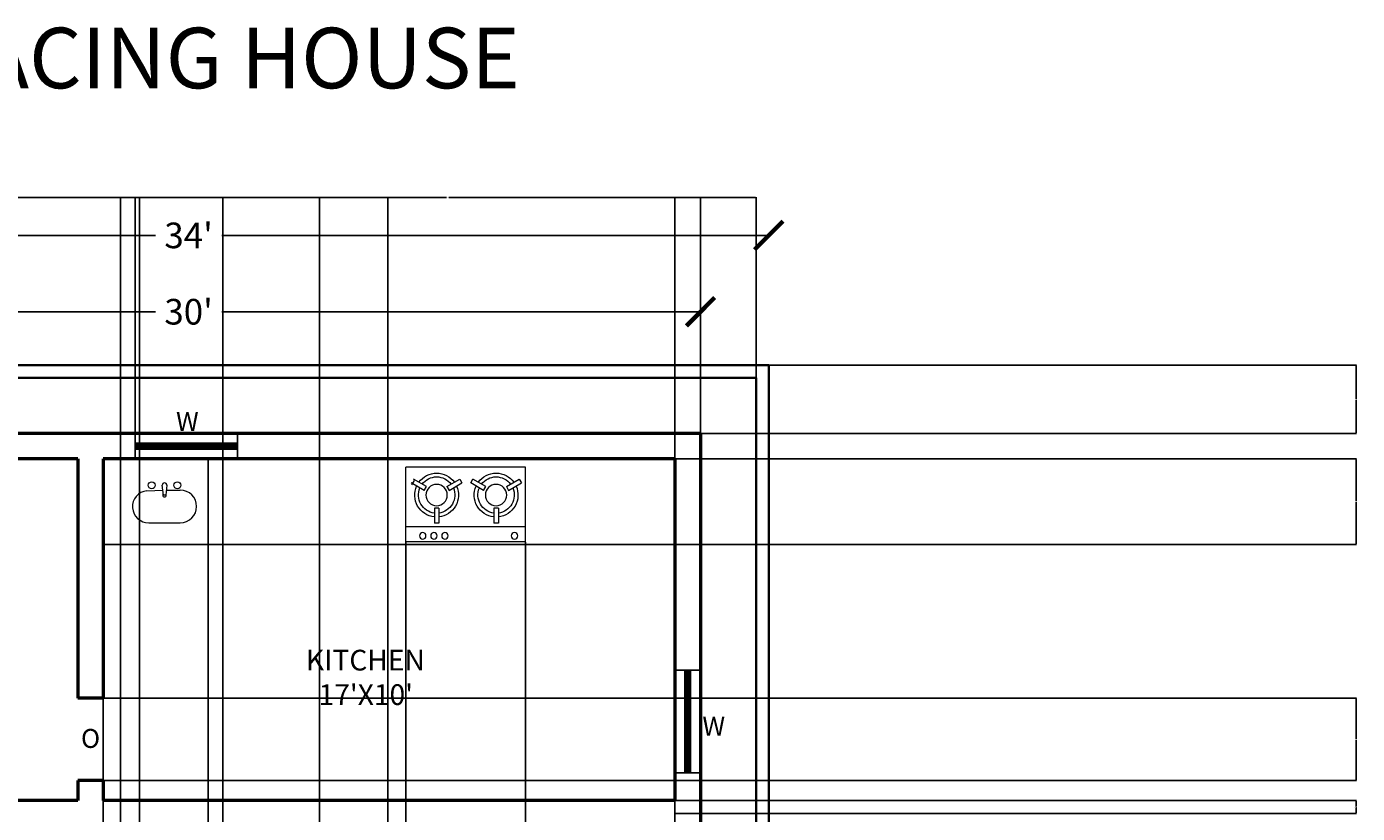
# Model space of a CAD drawing. Units: inches. Extents: x 338 to 1188, y -996 to 127.
# Tile 15 of 15: x 720 to 1188, y -149 to 127. Entities that reach past the tile are written whole.
import ezdxf

# ---------------------------------------------------------------- set-up
doc = ezdxf.new("R2010")
doc.units = ezdxf.units.IN
doc.header["$MEASUREMENT"] = 0
for name, color, linetype, lineweight in [('A-ANNO-DIMS', 5, 'Continuous', 18), ('A-ANNO-TEXT', 7, 'Continuous', 18), ('A-ANNO-TITL', 7, 'Continuous', 35), ('A-AREA-IDEN', 8, 'Continuous', 18), ('A-EQPM', 8, 'Continuous', 18), ('A-FLOR-CASE', 8, 'Continuous', 25), ('A-FLOR-FIXT', 8, 'Continuous', 18), ('A-GLAZ-PATT', 5, 'Continuous', 13), ('C-PROP', 1, 'Continuous', 35), ('wall', 1, 'Continuous', 50), ('win', 5, 'Continuous', 25)]:
    doc.layers.add(name, color=color, linetype=linetype, lineweight=lineweight)
doc.styles.get("Standard").update_dxf_attribs({"font": 'arial.ttf'})
doc.dimstyles.get("Standard").update_dxf_attribs({"dimtxt": 0.18, "dimasz": 0.18, "dimexe": 0.18, "dimexo": 0.0625, "dimgap": 0.09, "dimtad": 0, "dimtih": 1, "dimtoh": 1, "dimdec": 1, "dimzin": 0, "dimdsep": 46, "dimlunit": 4, "dimtxsty": 'Standard', "dimcen": 0.09, "dimadec": 0, "dimazin": 0, "dimtfac": 1, "dimtdec": 1, "dimtofl": 0, "dimtmove": 0, "dimatfit": 3, "dimfxl": 1, "dimtolj": 1, "dimtzin": 0, "dimarcsym": 0})

# ---------------------------------------------------------------- blocks, each defined once
blk = doc.blocks.new('_ArchTick')
at = {"color": 0, "linetype": 'ByBlock', "const_width": 0.15}
blk.add_lwpolyline([(-0.5, -0.5), (0.5, 0.5)], dxfattribs=at)
blk = doc.blocks.new('*D4')
at = {"layer": 'A-ANNO-DIMS', "color": 0, "lineweight": -2, "transparency": 16777216}
for p, q in [((596.96, 26.99), (765.33, 26.99)), ((956.96, 26.99), (788.6, 26.99))]:
    blk.add_line(p, q, dxfattribs=at)
at = {"layer": 'Defpoints', "color": 0, "transparency": 16777216}
for p in [(956.96, 26.99), (596.96, -15.73), (956.96, -15.73)]:
    blk.add_point(p, dxfattribs=at)
at = {"layer": 'A-ANNO-DIMS', "color": 0, "lineweight": -2, "transparency": 16777216, "xscale": 10, "yscale": 10, "zscale": 10, "rotation": 180}
blk.add_blockref('_ArchTick', (596.96, 26.99), dxfattribs=at)
at = {"layer": 'A-ANNO-DIMS', "color": 0, "lineweight": -2, "transparency": 16777216, "xscale": 10, "yscale": 10, "zscale": 10}
blk.add_blockref('_ArchTick', (956.96, 26.99), dxfattribs=at)
at = {"layer": 'A-ANNO-DIMS', "color": 0, "transparency": 16777216, "insert": (776.96, 26.99), "char_height": 9, "attachment_point": 5}
blk.add_mtext("\\A1;30'", dxfattribs=at)
blk = doc.blocks.new('*D5')
at = {"layer": 'A-ANNO-DIMS', "color": 0, "lineweight": -2, "transparency": 16777216}
for p, q in [((572.96, 53.81), (765.33, 53.81)), ((980.96, 53.81), (788.6, 53.81))]:
    blk.add_line(p, q, dxfattribs=at)
at = {"layer": 'Defpoints', "color": 0, "transparency": 16777216}
for p in [(980.96, 53.81), (572.96, 8.27), (980.96, 8.27)]:
    blk.add_point(p, dxfattribs=at)
at = {"layer": 'A-ANNO-DIMS', "color": 0, "lineweight": -2, "transparency": 16777216, "xscale": 10, "yscale": 10, "zscale": 10, "rotation": 180}
blk.add_blockref('_ArchTick', (572.96, 53.81), dxfattribs=at)
at = {"layer": 'A-ANNO-DIMS', "color": 0, "lineweight": -2, "transparency": 16777216, "xscale": 10, "yscale": 10, "zscale": 10}
blk.add_blockref('_ArchTick', (980.96, 53.81), dxfattribs=at)
at = {"layer": 'A-ANNO-DIMS', "color": 0, "transparency": 16777216, "insert": (776.96, 53.81), "char_height": 9, "attachment_point": 5}
blk.add_mtext("\\A1;34'", dxfattribs=at)
blk = doc.blocks.new('*D25')
at = {"layer": 'A-ANNO-DIMS', "color": 0, "lineweight": -2, "transparency": 16777216}
for p, q in [((981.03, 8.27), (1187.6, 8.27)), ((1187.42, 8.09), (1187.42, -3.55)), ((1187.42, -15.55), (1187.42, -3.91)), ((957.03, -15.73), (1187.6, -15.73))]:
    blk.add_line(p, q, dxfattribs=at)
at = {"layer": 'A-ANNO-DIMS', "color": 0, "transparency": 16777216}
for points in [[(1187.39, 8.09), (1187.45, 8.09), (1187.42, 8.27)], [(1187.39, -15.55), (1187.45, -15.55), (1187.42, -15.73)]]:
    blk.add_solid(points, dxfattribs=at)
at = {"layer": 'Defpoints', "color": 0, "transparency": 16777216}
for p in [(980.96, 8.27), (956.96, -15.73), (1187.42, -15.73)]:
    blk.add_point(p, dxfattribs=at)
at = {"layer": 'A-ANNO-DIMS', "color": 0, "transparency": 16777216, "insert": (1187.42, -3.73), "char_height": 0.18, "attachment_point": 5}
blk.add_mtext('\\A1;2\'-0"', dxfattribs=at)
blk = doc.blocks.new('*D30')
at = {"layer": 'A-ANNO-DIMS', "color": 0, "lineweight": -2, "transparency": 16777216}
for p, q in [((948.03, -24.73), (1187.6, -24.73)), ((1187.42, -24.91), (1187.42, -39.55)), ((1187.42, -54.55), (1187.42, -39.91)), ((948.03, -54.73), (1187.6, -54.73))]:
    blk.add_line(p, q, dxfattribs=at)
at = {"layer": 'A-ANNO-DIMS', "color": 0, "transparency": 16777216}
for points in [[(1187.39, -24.91), (1187.45, -24.91), (1187.42, -24.73)], [(1187.39, -54.55), (1187.45, -54.55), (1187.42, -54.73)]]:
    blk.add_solid(points, dxfattribs=at)
at = {"layer": 'Defpoints', "color": 0, "transparency": 16777216}
for p in [(947.96, -24.73), (947.96, -54.73), (1187.42, -54.73)]:
    blk.add_point(p, dxfattribs=at)
at = {"layer": 'A-ANNO-DIMS', "color": 0, "transparency": 16777216, "insert": (1187.42, -39.73), "char_height": 0.18, "attachment_point": 5}
blk.add_mtext('\\A1;2\'-6"', dxfattribs=at)
blk = doc.blocks.new('*D32')
at = {"layer": 'A-ANNO-DIMS', "color": 0, "lineweight": -2, "transparency": 16777216}
for p, q in [((738.03, -108.73), (1187.6, -108.73)), ((1187.42, -108.91), (1187.42, -123.05)), ((1187.42, -137.55), (1187.42, -123.41)), ((738.03, -137.73), (1187.6, -137.73))]:
    blk.add_line(p, q, dxfattribs=at)
at = {"layer": 'A-ANNO-DIMS', "color": 0, "transparency": 16777216}
for points in [[(1187.39, -108.91), (1187.45, -108.91), (1187.42, -108.73)], [(1187.39, -137.55), (1187.45, -137.55), (1187.42, -137.73)]]:
    blk.add_solid(points, dxfattribs=at)
at = {"layer": 'Defpoints', "color": 0, "transparency": 16777216}
for p in [(737.96, -108.73), (737.96, -137.73), (1187.42, -137.73)]:
    blk.add_point(p, dxfattribs=at)
at = {"layer": 'A-ANNO-DIMS', "color": 0, "transparency": 16777216, "insert": (1187.42, -123.23), "char_height": 0.18, "attachment_point": 5}
blk.add_mtext('\\A1;2\'-5"', dxfattribs=at)
blk = doc.blocks.new('*D37')
at = {"layer": 'A-ANNO-DIMS', "color": 0, "lineweight": -2, "transparency": 16777216}
for p, q in [((752.96, -393.67), (752.96, 67.25)), ((753.14, 67.07), (770.63, 67.07)), ((788.78, 67.07), (771.29, 67.07)), ((788.96, -393.67), (788.96, 67.25))]:
    blk.add_line(p, q, dxfattribs=at)
at = {"layer": 'A-ANNO-DIMS', "color": 0, "transparency": 16777216}
for points in [[(753.14, 67.1), (753.14, 67.04), (752.96, 67.07)], [(788.78, 67.1), (788.78, 67.04), (788.96, 67.07)]]:
    blk.add_solid(points, dxfattribs=at)
at = {"layer": 'Defpoints', "color": 0, "transparency": 16777216}
for p in [(788.96, 67.07), (752.96, -393.73), (788.96, -393.73)]:
    blk.add_point(p, dxfattribs=at)
at = {"layer": 'A-ANNO-DIMS', "color": 0, "transparency": 16777216, "insert": (770.96, 67.07), "char_height": 0.18, "attachment_point": 5}
blk.add_mtext('\\A1;3\'-0"', dxfattribs=at)
blk = doc.blocks.new('*D38')
at = {"layer": 'A-ANNO-DIMS', "color": 0, "lineweight": -2, "transparency": 16777216}
for p, q in [((822.96, -470.17), (822.96, 67.25)), ((823.14, 67.07), (834.63, 67.07)), ((846.78, 67.07), (835.29, 67.07)), ((846.96, -470.17), (846.96, 67.25))]:
    blk.add_line(p, q, dxfattribs=at)
at = {"layer": 'A-ANNO-DIMS', "color": 0, "transparency": 16777216}
for points in [[(823.14, 67.1), (823.14, 67.04), (822.96, 67.07)], [(846.78, 67.1), (846.78, 67.04), (846.96, 67.07)]]:
    blk.add_solid(points, dxfattribs=at)
at = {"layer": 'Defpoints', "color": 0, "transparency": 16777216}
for p in [(846.96, 67.07), (822.96, -470.23), (846.96, -470.23)]:
    blk.add_point(p, dxfattribs=at)
at = {"layer": 'A-ANNO-DIMS', "color": 0, "transparency": 16777216, "insert": (834.96, 67.07), "char_height": 0.18, "attachment_point": 5}
blk.add_mtext('\\A1;2\'-0"', dxfattribs=at)
blk = doc.blocks.new('*D42')
at = {"layer": 'A-ANNO-DIMS', "color": 0, "lineweight": -2, "transparency": 16777216}
for p, q in [((746.96, -54.8), (746.96, -968.86)), ((783.89, -54.8), (783.89, -968.86)), ((747.14, -968.68), (765.1, -968.68)), ((783.71, -968.68), (765.76, -968.68))]:
    blk.add_line(p, q, dxfattribs=at)
at = {"layer": 'A-ANNO-DIMS', "color": 0, "transparency": 16777216}
for points in [[(747.14, -968.65), (747.14, -968.71), (746.96, -968.68)], [(783.71, -968.65), (783.71, -968.71), (783.89, -968.68)]]:
    blk.add_solid(points, dxfattribs=at)
at = {"layer": 'Defpoints', "color": 0, "transparency": 16777216}
for p in [(746.96, -54.73), (783.89, -54.73), (783.89, -968.68)]:
    blk.add_point(p, dxfattribs=at)
at = {"layer": 'A-ANNO-DIMS', "color": 0, "transparency": 16777216, "insert": (765.43, -968.68), "char_height": 0.18, "attachment_point": 5}
blk.add_mtext('\\A1;3\'-1"', dxfattribs=at)
blk = doc.blocks.new('*D43')
at = {"layer": 'A-ANNO-DIMS', "color": 0, "lineweight": -2, "transparency": 16777216}
for p, q in [((853.28, -53.93), (853.28, -968.86)), ((895.37, -53.93), (895.37, -968.86)), ((853.46, -968.68), (873.99, -968.68)), ((895.19, -968.68), (874.65, -968.68))]:
    blk.add_line(p, q, dxfattribs=at)
at = {"layer": 'A-ANNO-DIMS', "color": 0, "transparency": 16777216}
for points in [[(853.46, -968.65), (853.46, -968.71), (853.28, -968.68)], [(895.19, -968.65), (895.19, -968.71), (895.37, -968.68)]]:
    blk.add_solid(points, dxfattribs=at)
at = {"layer": 'Defpoints', "color": 0, "transparency": 16777216}
for p in [(853.28, -53.87), (895.37, -53.87), (895.37, -968.68)]:
    blk.add_point(p, dxfattribs=at)
at = {"layer": 'A-ANNO-DIMS', "color": 0, "transparency": 16777216, "insert": (874.32, -968.68), "char_height": 0.18, "attachment_point": 5}
blk.add_mtext('\\A1;3\'-6"', dxfattribs=at)
blk = doc.blocks.new('*D44')
at = {"layer": 'A-ANNO-DIMS', "color": 0, "lineweight": -2, "transparency": 16777216}
for p, q in [((895.37, -53.93), (895.37, -968.86)), ((947.96, -54.8), (947.96, -968.86)), ((895.55, -968.68), (921.12, -968.68)), ((947.78, -968.68), (922.21, -968.68))]:
    blk.add_line(p, q, dxfattribs=at)
at = {"layer": 'A-ANNO-DIMS', "color": 0, "transparency": 16777216}
for points in [[(895.55, -968.65), (895.55, -968.71), (895.37, -968.68)], [(947.78, -968.65), (947.78, -968.71), (947.96, -968.68)]]:
    blk.add_solid(points, dxfattribs=at)
at = {"layer": 'Defpoints', "color": 0, "transparency": 16777216}
for p in [(895.37, -53.87), (947.96, -54.73), (947.96, -968.68)]:
    blk.add_point(p, dxfattribs=at)
at = {"layer": 'A-ANNO-DIMS', "color": 0, "transparency": 16777216, "insert": (921.67, -968.68), "char_height": 0.18, "attachment_point": 5}
blk.add_mtext('\\A1;4\'-4 1/2"', dxfattribs=at)
blk = doc.blocks.new('*D45')
at = {"layer": 'A-ANNO-DIMS', "color": 0, "lineweight": -2, "transparency": 16777216}
for p, q in [((947.96, -24.67), (947.96, 67.25)), ((948.14, 67.07), (952.13, 67.07)), ((956.78, 67.07), (952.79, 67.07)), ((956.96, -15.67), (956.96, 67.25))]:
    blk.add_line(p, q, dxfattribs=at)
at = {"layer": 'A-ANNO-DIMS', "color": 0, "transparency": 16777216}
for points in [[(948.14, 67.1), (948.14, 67.04), (947.96, 67.07)], [(956.78, 67.1), (956.78, 67.04), (956.96, 67.07)]]:
    blk.add_solid(points, dxfattribs=at)
at = {"layer": 'Defpoints', "color": 0, "transparency": 16777216}
for p in [(956.96, 67.07), (956.96, -15.73), (947.96, -24.73)]:
    blk.add_point(p, dxfattribs=at)
at = {"layer": 'A-ANNO-DIMS', "color": 0, "transparency": 16777216, "insert": (952.46, 67.07), "char_height": 0.18, "attachment_point": 5}
blk.add_mtext('\\A1;0\'-9"', dxfattribs=at)
blk = doc.blocks.new('*D46')
at = {"layer": 'A-ANNO-DIMS', "color": 0, "lineweight": -2, "transparency": 16777216}
for p, q in [((948.03, -144.73), (1187.6, -144.73)), ((1187.42, -144.91), (1187.42, -146.8)), ((948.03, -149.23), (1187.6, -149.23)), ((1187.42, -149.05), (1187.42, -147.17))]:
    blk.add_line(p, q, dxfattribs=at)
at = {"layer": 'A-ANNO-DIMS', "color": 0, "transparency": 16777216}
for points in [[(1187.39, -144.91), (1187.45, -144.91), (1187.42, -144.73)], [(1187.39, -149.05), (1187.45, -149.05), (1187.42, -149.23)]]:
    blk.add_solid(points, dxfattribs=at)
at = {"layer": 'Defpoints', "color": 0, "transparency": 16777216}
for p in [(947.96, -144.73), (947.96, -149.23), (1187.42, -149.23)]:
    blk.add_point(p, dxfattribs=at)
at = {"layer": 'A-ANNO-DIMS', "color": 0, "transparency": 16777216, "insert": (1187.42, -146.98), "char_height": 0.18, "attachment_point": 5}
blk.add_mtext('\\A1;0\'-4 1/2"', dxfattribs=at)
blk = doc.blocks.new('*D47')
at = {"layer": 'A-ANNO-DIMS', "color": 0, "lineweight": -2, "transparency": 16777216}
for p, q in [((759.67, -755.17), (759.67, 67.25)), ((759.85, 67.07), (867.68, 67.07)), ((976.28, 67.07), (868.46, 67.07)), ((976.46, -755.17), (976.46, 67.25))]:
    blk.add_line(p, q, dxfattribs=at)
at = {"layer": 'A-ANNO-DIMS', "color": 0, "transparency": 16777216}
for points in [[(759.85, 67.1), (759.85, 67.04), (759.67, 67.07)], [(976.28, 67.1), (976.28, 67.04), (976.46, 67.07)]]:
    blk.add_solid(points, dxfattribs=at)
at = {"layer": 'Defpoints', "color": 0, "transparency": 16777216}
for p in [(976.46, 67.07), (759.67, -755.23), (976.46, -755.23)]:
    blk.add_point(p, dxfattribs=at)
at = {"layer": 'A-ANNO-DIMS', "color": 0, "transparency": 16777216, "insert": (868.07, 67.07), "char_height": 0.18, "attachment_point": 5}
blk.add_mtext('\\A1;18\'-1"', dxfattribs=at)
blk = doc.blocks.new('*D50')
at = {"layer": 'A-ANNO-DIMS', "color": 0, "lineweight": -2, "transparency": 16777216}
for p, q in [((668.69, -15.67), (668.69, 67.25)), ((668.87, 67.07), (712.91, 67.07)), ((758.03, 67.07), (713.99, 67.07)), ((758.21, -15.67), (758.21, 67.25))]:
    blk.add_line(p, q, dxfattribs=at)
at = {"layer": 'A-ANNO-DIMS', "color": 0, "transparency": 16777216}
for points in [[(668.87, 67.1), (668.87, 67.04), (668.69, 67.07)], [(758.03, 67.1), (758.03, 67.04), (758.21, 67.07)]]:
    blk.add_solid(points, dxfattribs=at)
at = {"layer": 'Defpoints', "color": 0, "transparency": 16777216}
for p in [(758.21, 67.07), (668.69, -15.73), (758.21, -15.73)]:
    blk.add_point(p, dxfattribs=at)
at = {"layer": 'A-ANNO-DIMS', "color": 0, "transparency": 16777216, "insert": (713.45, 67.07), "char_height": 0.18, "attachment_point": 5}
blk.add_mtext('\\A1;7\'-5 1/2"', dxfattribs=at)

msp = doc.modelspace()

# ---------------------------------------------------------------- hatches: boundary and pattern name
at = {"layer": 'A-GLAZ-PATT'}
h = msp.add_hatch(dxfattribs=at)
h.set_pattern_fill('ANSI31', color=256)
h.paths.add_polyline_path([(953.46, -405.07), (951.46, -405.07), (951.46, -429.07), (953.46, -429.07)])
h.paths.add_polyline_path([(953.46, -485.22), (951.46, -485.22), (951.46, -521.22), (953.46, -521.22)])
h.paths.add_polyline_path([(794.21, -19.23), (758.21, -19.23), (758.21, -21.23), (794.21, -21.23)])
h.paths.add_polyline_path([(668.69, -19.23), (632.69, -19.23), (632.69, -21.23), (668.69, -21.23)])
h.paths.add_polyline_path([(602.46, -94.89), (600.46, -94.89), (600.46, -130.89), (602.46, -130.89)])
h.paths.add_polyline_path([(602.46, -243.73), (600.46, -243.73), (600.46, -315.73), (602.46, -315.73)])
h = msp.add_hatch(dxfattribs=at)
h.set_pattern_fill('ANSI31', color=256)
h.paths.add_polyline_path([(953.46, -98.96), (951.46, -98.96), (951.46, -134.96), (953.46, -134.96)])
h.paths.add_polyline_path([(953.46, -163.12), (951.46, -163.12), (951.46, -187.12), (953.46, -187.12)])
h.paths.add_polyline_path([(953.46, -227.22), (951.46, -227.22), (951.46, -297.73), (953.46, -297.73)])

# ---------------------------------------------------------------- linework, layer by layer
at = {"layer": 'A-EQPM'}
for p, q in [((895.37, -27.57), (853.28, -27.57)), ((853.28, -53.87), (853.28, -27.57)), ((895.37, -53.87), (895.37, -27.57)), ((855.45, -33.78), (856.33, -32.26)), ((860.56, -34.42), (856.02, -31.8)), ((867.75, -34.42), (872.29, -31.8)), ((872.29, -31.8), (873.08, -33.17)), ((876.15, -33.16), (876.94, -31.8)), ((881.48, -34.42), (876.94, -31.8)), ((888.67, -34.42), (893.21, -31.8)), ((893.21, -31.8), (894, -33.17)), ((859.77, -35.79), (855.23, -33.16)), ((859.77, -35.79), (860.56, -34.42)), ((867.75, -34.42), (868.54, -35.79)), ((868.54, -35.79), (873.08, -33.17)), ((880.69, -35.79), (876.15, -33.16)), ((880.69, -35.79), (881.48, -34.42)), ((888.67, -34.42), (889.46, -35.79)), ((889.46, -35.79), (894, -33.17)), ((863.37, -42.01), (863.36, -47.26)), ((864.94, -42.01), (863.37, -42.01)), ((864.94, -42.01), (864.94, -47.26)), ((884.28, -42.01), (884.28, -47.26)), ((885.86, -42.01), (884.28, -42.01)), ((885.86, -42.01), (885.86, -47.26)), ((895.37, -48.61), (853.28, -48.61)), ((864.94, -47.26), (863.36, -47.26)), ((885.86, -47.26), (884.28, -47.26)), ((895.37, -53.87), (853.28, -53.87))]:
    msp.add_line(p, q, dxfattribs=at)
at = {"layer": 'A-EQPM', "extrusion": (0, 0, -1)}
for centre, major_axis, start_param, end_param in [((864.16, -37.41), (-0.01, 7.71), -0.942584, 0.946692), ((864.16, -37.41), (-4.52, 4.52), 6.145519, 7.992397), ((885.07, -37.41), (0, 7.71), -0.944011, 0.945266), ((885.07, -37.41), (-4.52, 4.52), 6.145519, 7.992397), ((864.16, -37.41), (0, 7.71), 3.2451, 5.134376), ((864.16, -37.41), (-4.52, 4.52), 4.051123, 5.898002), ((864.16, -37.41), (-2.66, 2.66), 2.356194490192312, 8.639379797371898), ((864.16, -37.41), (0.01, 7.71), 1.148752, 3.038029), ((864.16, -37.41), (4.52, 4.52), 0.385932, 2.23281), ((885.07, -37.41), (0, 7.71), 3.244173, 5.13345), ((885.07, -37.41), (4.52, 4.52), 2.480327, 4.327205), ((885.07, -37.41), (-2.66, 2.66), 2.356194490192306, 8.639379797371893), ((885.07, -37.41), (0.01, 7.71), 1.14879, 3.038067), ((885.07, -37.41), (4.52, 4.52), 0.385932, 2.23281), ((859.27, -51.72), (-0.807, 0.807), 2.35619449019219, 8.639379797371777), ((863.22, -51.72), (-0.807, 0.807), 2.35619449019219, 8.639379797371777), ((867.09, -51.72), (-0.807, 0.807), 2.35619449019219, 8.639379797371777), ((891.52, -51.72), (-0.807, 0.807), 2.35619449019219, 8.639379797371777)]:
    msp.add_ellipse(centre, major_axis=major_axis, ratio=1, start_param=start_param, end_param=end_param, dxfattribs=at)
at = {"layer": 'A-FLOR-CASE'}
for p, q in [((783.89, -54.73), (783.89, -24.73)), ((947.96, -54.73), (746.96, -54.73))]:
    msp.add_line(p, q, dxfattribs=at)
at = {"layer": 'A-FLOR-FIXT'}
for p, q in [((762.26, -35.88), (767.89, -35.72)), ((768.09, -37.47), (767.68, -33.98)), ((769.32, -33.98), (768.91, -37.47)), ((769.12, -35.67), (774.04, -35.67)), ((768.97, -37.47), (768.09, -37.47)), ((762.97, -47.15), (774.04, -47.15))]:
    msp.add_line(p, q, dxfattribs=at)
for centre in [(763.99, -33.98), (773.01, -33.98)]:
    msp.add_circle(centre, 1.23, dxfattribs=at)
for centre, radius, start, end in [((762.88, -41.5), 5.65, 96.3659, 270.8792), ((768.5, -33.98), 0.82, 0, 180), ((768.5, -37.47), 0.615, 138.1701, 41.8299), ((774.04, -41.41), 5.74, 270, 90)]:
    msp.add_arc(centre, radius, start, end, dxfattribs=at)
at = {"layer": 'C-PROP'}
for p, q in [((980.96, 8.27), (572.96, 8.27)), ((980.96, 8.27), (980.96, -807.73)), ((976.46, 3.77), (577.46, 3.77)), ((976.46, 3.77), (976.46, -803.23))]:
    msp.add_line(p, q, dxfattribs=at)
at = {"layer": 'wall'}
for p, q in [((956.96, -15.73), (596.96, -15.73)), ((956.96, -15.73), (956.96, -615.73)), ((737.96, -24.73), (605.96, -24.73)), ((737.96, -24.73), (737.96, -108.73)), ((737.96, -24.73), (737.96, -108.73)), ((947.96, -24.73), (746.96, -24.73)), ((746.96, -24.73), (746.96, -108.73)), ((947.96, -24.73), (947.96, -144.73)), ((746.96, -108.73), (737.96, -108.73)), ((746.96, -137.73), (737.96, -137.73)), ((737.96, -137.73), (737.96, -144.73)), ((737.96, -137.73), (737.96, -144.73)), ((746.96, -137.73), (746.96, -144.73)), ((737.96, -144.73), (701.96, -144.73)), ((947.96, -144.73), (746.96, -144.73))]:
    msp.add_line(p, q, dxfattribs=at)
at = {"layer": 'win'}
for p, q in [((758.21, -24.73), (758.21, -15.73)), ((794.21, -24.73), (794.21, -15.73)), ((758.21, -19.23), (794.21, -19.23)), ((758.21, -21.23), (794.21, -21.23)), ((947.96, -98.96), (956.96, -98.96)), ((951.46, -98.96), (951.46, -134.96)), ((953.46, -98.96), (953.46, -134.96)), ((947.96, -134.96), (956.96, -134.96))]:
    msp.add_line(p, q, dxfattribs=at)

# ---------------------------------------------------------------- texts
at = {"layer": 'A-ANNO-TEXT'}
for s, p in [('W', (772.54, -14.86)), ('W', (957.61, -121.96)), ('O', (739.12, -126.24))]:
    msp.add_text(s, height=6.65, dxfattribs=at).set_placement(p)
at = {"layer": 'A-ANNO-TITL', "insert": (603.41, 126.77), "char_height": 21.2807, "attachment_point": 1}
msp.add_mtext_dynamic_manual_height_columns('WEST FACING HOUSE', width=345.7385, gutter_width=3.55, heights=[0], dxfattribs=at)
at = {"layer": 'A-AREA-IDEN', "insert": (809.32, -91.77), "char_height": 7.2703, "attachment_point": 1}
msp.add_mtext_dynamic_manual_height_columns("    KITCHEN\\P      17'X10'", width=65.8887, gutter_width=1.21, heights=[0], dxfattribs=at)

# ---------------------------------------------------------------- dimensions: what is measured, and where the dimension line sits
at = {"layer": 'A-ANNO-DIMS'}
for base, p1, p2, override, picture, middle in [((758.21, 67.07), (668.69, -15.73), (758.21, -15.73), {"dimdec": 1, "dimlfac": 1, "dimrnd": 0, "dimzin": 1, "dimdsep": 46, "dimlunit": 4, "dimfrac": 2}, '*D50', (713.45, 67.07)), ((788.96, 67.07), (752.96, -393.73), (788.96, -393.73), {"dimdec": 1, "dimlfac": 1, "dimrnd": 0, "dimzin": 1, "dimdsep": 46, "dimlunit": 4, "dimfrac": 2}, '*D37', (770.96, 67.07)), ((976.46, 67.07), (759.67, -755.23), (976.46, -755.23), {"dimdec": 1, "dimlfac": 1, "dimrnd": 0, "dimzin": 1, "dimdsep": 46, "dimlunit": 4, "dimfrac": 2}, '*D47', (868.07, 67.07)), ((846.96, 67.07), (822.96, -470.23), (846.96, -470.23), {"dimdec": 1, "dimlfac": 1, "dimrnd": 0, "dimzin": 1, "dimdsep": 46, "dimlunit": 4, "dimfrac": 2}, '*D38', (834.96, 67.07)), ((956.96, 67.07), (947.96, -24.73), (956.96, -15.73), {"dimdec": 1, "dimlfac": 1, "dimrnd": 0, "dimzin": 1, "dimdsep": 46, "dimlunit": 4, "dimfrac": 2}, '*D45', (952.46, 67.07)), ((980.96, 53.81), (572.96, 8.27), (980.96, 8.27), {"dimtxt": 9, "dimasz": 10, "dimgap": 4, "dimblk1": 'ArchTick', "dimblk2": 'ArchTick', "dimsah": 1, "dimse1": 1, "dimse2": 1, "dimclrd": 0, "dimclre": 0, "dimclrt": 0}, '*D5', (776.96, 53.81)), ((956.96, 26.99), (596.96, -15.73), (956.96, -15.73), {"dimtxt": 9, "dimasz": 10, "dimgap": 4, "dimblk1": 'ArchTick', "dimblk2": 'ArchTick', "dimsah": 1, "dimse1": 1, "dimse2": 1, "dimclrd": 0, "dimclre": 0, "dimclrt": 0}, '*D4', (776.96, 26.99)), ((783.89, -968.68), (746.96, -54.73), (783.89, -54.73), {"dimdec": 1, "dimlfac": 1, "dimrnd": 0, "dimzin": 1, "dimdsep": 46, "dimlunit": 4, "dimfrac": 2}, '*D42', (765.43, -968.68)), ((895.37, -968.68), (853.28, -53.87), (895.37, -53.87), {"dimdec": 1, "dimlfac": 1, "dimrnd": 0, "dimzin": 1, "dimdsep": 46, "dimlunit": 4, "dimfrac": 2}, '*D43', (874.32, -968.68)), ((947.96, -968.68), (895.37, -53.87), (947.96, -54.73), {"dimdec": 1, "dimlfac": 1, "dimrnd": 0, "dimzin": 1, "dimdsep": 46, "dimlunit": 4, "dimfrac": 2}, '*D44', (921.67, -968.68))]:
    dim = msp.add_linear_dim(base=base, p1=p1, p2=p2, dimstyle='Standard', override=override, dxfattribs=at)
    dim.commit()
    dim.dimension.update_dxf_attribs({"geometry": picture, "text_midpoint": middle})
for base, p1, p2, picture, middle in [((1187.42, -15.73), (980.96, 8.27), (956.96, -15.73), '*D25', (1187.42, -3.73)), ((1187.42, -54.73), (947.96, -24.73), (947.96, -54.73), '*D30', (1187.42, -39.73)), ((1187.42, -137.73), (737.96, -108.73), (737.96, -137.73), '*D32', (1187.42, -123.23)), ((1187.42, -149.23), (947.96, -144.73), (947.96, -149.23), '*D46', (1187.42, -146.98))]:
    dim = msp.add_linear_dim(base=base, p1=p1, p2=p2, angle=90, dimstyle='Standard', override={"dimdec": 1, "dimlfac": 1, "dimrnd": 0, "dimzin": 1, "dimdsep": 46, "dimlunit": 4, "dimfrac": 2}, dxfattribs=at)
    dim.commit()
    dim.dimension.update_dxf_attribs({"geometry": picture, "text_midpoint": middle})

doc.saveas('drawing.dxf')
